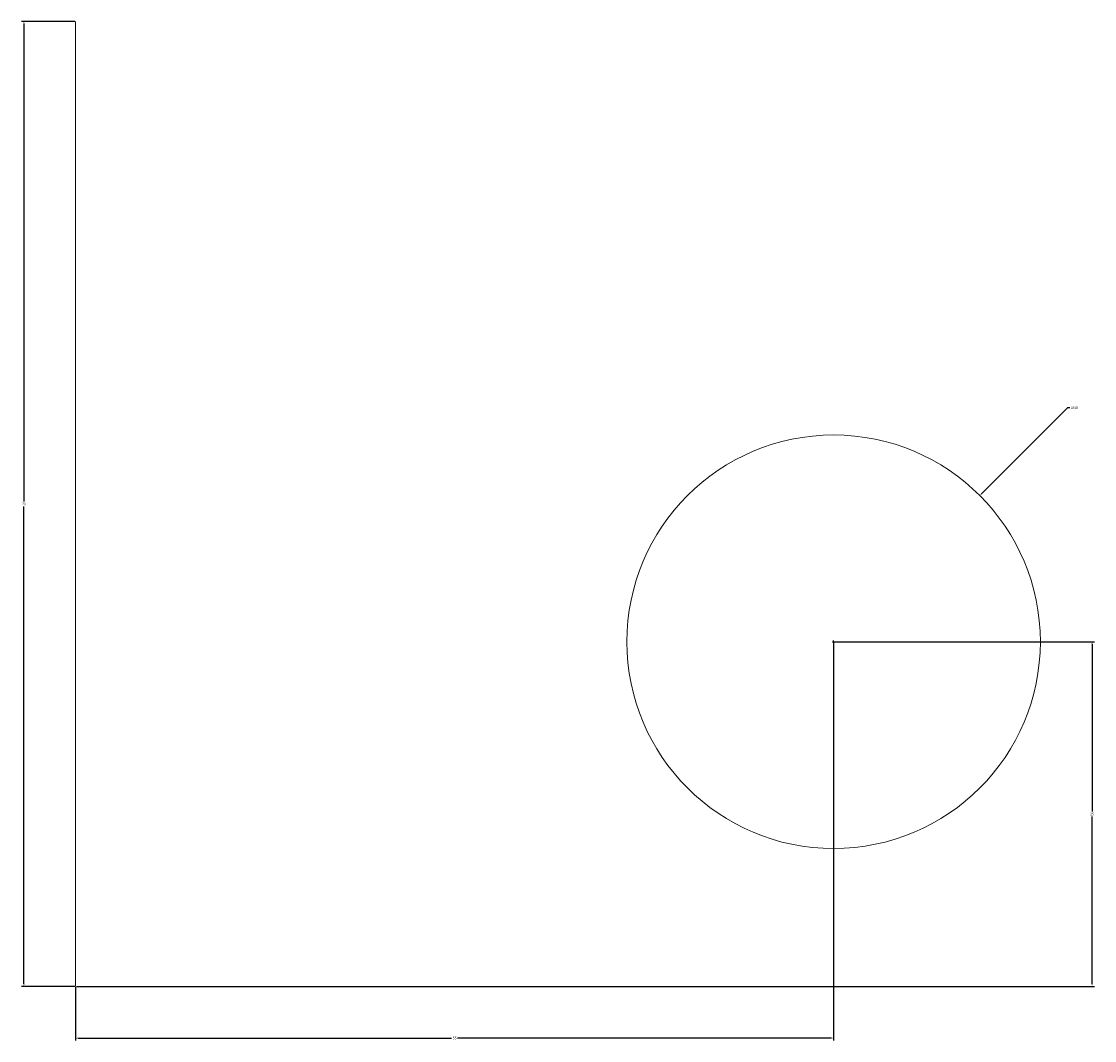
# Model space of a CAD drawing. Units: millimetres. Extents: x -3.9 to 73.9, y 1420.4 to 1494.3.
import ezdxf

# ---------------------------------------------------------------- set-up
doc = ezdxf.new("R2010")
doc.units = ezdxf.units.MM
doc.layers.add('M-CONS', color=8, linetype='Continuous', lineweight=18)
doc.layers.add('M-DIMS', color=2, linetype='Continuous', lineweight=18)
doc.styles.get("Standard").update_dxf_attribs({"font": 'arial.ttf'})
doc.dimstyles.get("Standard").update_dxf_attribs({"dimtxt": 0.18, "dimasz": 0.18, "dimexe": 0.18, "dimexo": 0.0625, "dimgap": 0.09, "dimtad": 0, "dimtih": 1, "dimtoh": 1, "dimdec": 4, "dimzin": 0, "dimdsep": 46, "dimtxsty": 'Standard', "dimcen": 0.09, "dimadec": 0, "dimazin": 0, "dimtfac": 1, "dimtdec": 4, "dimtofl": 0, "dimtmove": 0, "dimatfit": 3, "dimfxl": 1, "dimtolj": 1, "dimtzin": 0, "dimarcsym": 0})

# ---------------------------------------------------------------- blocks, each defined once
blk = doc.blocks.new('*D1')
at = {"layer": 'Defpoints', "color": 0, "transparency": 16777216}
for p in [(-3.75, 1494.297), (0, 1494.297), (0, 1424.297)]:
    blk.add_point(p, dxfattribs=at)
at = {"layer": 'M-DIMS', "color": 0, "lineweight": -2, "transparency": 16777216}
for p, q in [((-0.062, 1494.297), (-3.93, 1494.297)), ((-3.75, 1494.117), (-3.75, 1459.479)), ((-3.75, 1424.477), (-3.75, 1459.115)), ((-0.062, 1424.297), (-3.93, 1424.297))]:
    blk.add_line(p, q, dxfattribs=at)
at = {"layer": 'M-DIMS', "color": 0, "transparency": 16777216}
for points in [[(-3.78, 1494.117), (-3.72, 1494.117), (-3.75, 1494.297)], [(-3.78, 1424.477), (-3.72, 1424.477), (-3.75, 1424.297)]]:
    blk.add_solid(points, dxfattribs=at)
at = {"layer": 'M-DIMS', "color": 0, "transparency": 16777216, "insert": (-3.75, 1459.297), "char_height": 0.18, "attachment_point": 5}
blk.add_mtext('\\A1;70', dxfattribs=at)
blk = doc.blocks.new('*D2')
at = {"layer": 'Defpoints', "color": 0, "transparency": 16777216}
for p in [(55, 1449.297), (0, 1424.297), (55, 1420.547)]:
    blk.add_point(p, dxfattribs=at)
at = {"layer": 'M-DIMS', "color": 0, "lineweight": -2, "transparency": 16777216}
for p, q in [((55, 1449.235), (55, 1420.367)), ((0, 1424.235), (0, 1420.367)), ((0.18, 1420.547), (27.28, 1420.547)), ((54.82, 1420.547), (27.72, 1420.547))]:
    blk.add_line(p, q, dxfattribs=at)
at = {"layer": 'M-DIMS', "color": 0, "transparency": 16777216}
for points in [[(0.18, 1420.577), (0.18, 1420.517), (0, 1420.547)], [(54.82, 1420.577), (54.82, 1420.517), (55, 1420.547)]]:
    blk.add_solid(points, dxfattribs=at)
at = {"layer": 'M-DIMS', "color": 0, "transparency": 16777216, "insert": (27.5, 1420.547), "char_height": 0.18, "attachment_point": 5}
blk.add_mtext('\\A1;55', dxfattribs=at)
blk = doc.blocks.new('*D3')
at = {"layer": 'Defpoints', "color": 0, "transparency": 16777216}
for p in [(55, 1449.297), (73.75, 1449.297), (0, 1424.297)]:
    blk.add_point(p, dxfattribs=at)
at = {"layer": 'M-DIMS', "color": 0, "lineweight": -2, "transparency": 16777216}
for p, q in [((55.063, 1449.297), (73.93, 1449.297)), ((73.75, 1449.117), (73.75, 1436.979)), ((73.75, 1424.477), (73.75, 1436.615)), ((0.062, 1424.297), (73.93, 1424.297))]:
    blk.add_line(p, q, dxfattribs=at)
at = {"layer": 'M-DIMS', "color": 0, "transparency": 16777216}
for points in [[(73.72, 1449.117), (73.78, 1449.117), (73.75, 1449.297)], [(73.72, 1424.477), (73.78, 1424.477), (73.75, 1424.297)]]:
    blk.add_solid(points, dxfattribs=at)
at = {"layer": 'M-DIMS', "color": 0, "transparency": 16777216, "insert": (73.75, 1436.797), "char_height": 0.18, "attachment_point": 5}
blk.add_mtext('\\A1;25', dxfattribs=at)
blk = doc.blocks.new('*D4')
at = {"layer": 'Defpoints', "color": 0, "transparency": 16777216}
for p in [(65.605, 1459.905), (44.395, 1438.689)]:
    blk.add_point(p, dxfattribs=at)
at = {"layer": 'M-DIMS', "color": 0, "lineweight": -2, "transparency": 16777216}
for p, q in [((71.968, 1466.27), (65.732, 1460.032)), ((72.148, 1466.27), (71.968, 1466.27)), ((54.91, 1449.297), (55.09, 1449.297)), ((55, 1449.207), (55, 1449.387))]:
    blk.add_line(p, q, dxfattribs=at)
at = {"layer": 'M-DIMS', "color": 0, "transparency": 16777216}
blk.add_solid([(65.711, 1460.054), (65.754, 1460.011), (65.605, 1459.905)], dxfattribs=at)
at = {"layer": 'M-DIMS', "color": 0, "transparency": 16777216, "insert": (72.465, 1466.27), "char_height": 0.18, "attachment_point": 5}
blk.add_mtext('\\A1;∅30', dxfattribs=at)

msp = doc.modelspace()

# ---------------------------------------------------------------- linework, layer by layer
at = {"layer": 'M-CONS', "extrusion": (-1, 0, 0)}
msp.add_lwpolyline([(-1479.297, -24.561), (-1479.297, -9.561), (-1439.297, -9.561), (-1439.297, -24.561), (-1424.297, -24.561), (-1424.297, 5.439), (-1494.297, 5.439), (-1494.297, -24.561)], close=True, dxfattribs=at)
at = {"layer": 'M-CONS'}
msp.add_circle((55, 1449.297, 5.439), 15, dxfattribs=at)

# ---------------------------------------------------------------- dimensions: what is measured, and where the dimension line sits
at = {"layer": 'M-DIMS'}
for base, p2, picture, middle in [((-3.75, 1494.297), (0, 1494.297), '*D1', (-3.75, 1459.297)), ((73.75, 1449.297), (55, 1449.297), '*D3', (73.75, 1436.797))]:
    dim = msp.add_linear_dim(base=base, p1=(0, 1424.297), p2=p2, angle=90, dimstyle='Standard', override={"dimdec": 0, "dimlfac": 1, "dimrnd": 0, "dimzin": 0, "dimdsep": 46, "dimlunit": 2}, dxfattribs=at)
    dim.commit()
    dim.dimension.update_dxf_attribs({"geometry": picture, "text_midpoint": middle})
dim = msp.add_diameter_dim_2p(p1=(44.395, 1438.689), p2=(65.605, 1459.905), dimstyle='Standard', override={"dimdec": 0, "dimlfac": 1, "dimrnd": 0, "dimzin": 0, "dimdsep": 46, "dimlunit": 2}, dxfattribs=at)
dim.commit()
dim.dimension.update_dxf_attribs({"geometry": '*D4', "text_midpoint": (72.465, 1466.27), "dimtype": 163})
dim = msp.add_linear_dim(base=(55, 1420.547), p1=(0, 1424.297), p2=(55, 1449.297), dimstyle='Standard', override={"dimdec": 0, "dimlfac": 1, "dimrnd": 0, "dimzin": 0, "dimdsep": 46, "dimlunit": 2}, dxfattribs=at)
dim.commit()
dim.dimension.update_dxf_attribs({"geometry": '*D2', "text_midpoint": (27.5, 1420.547)})

doc.saveas('drawing.dxf')
